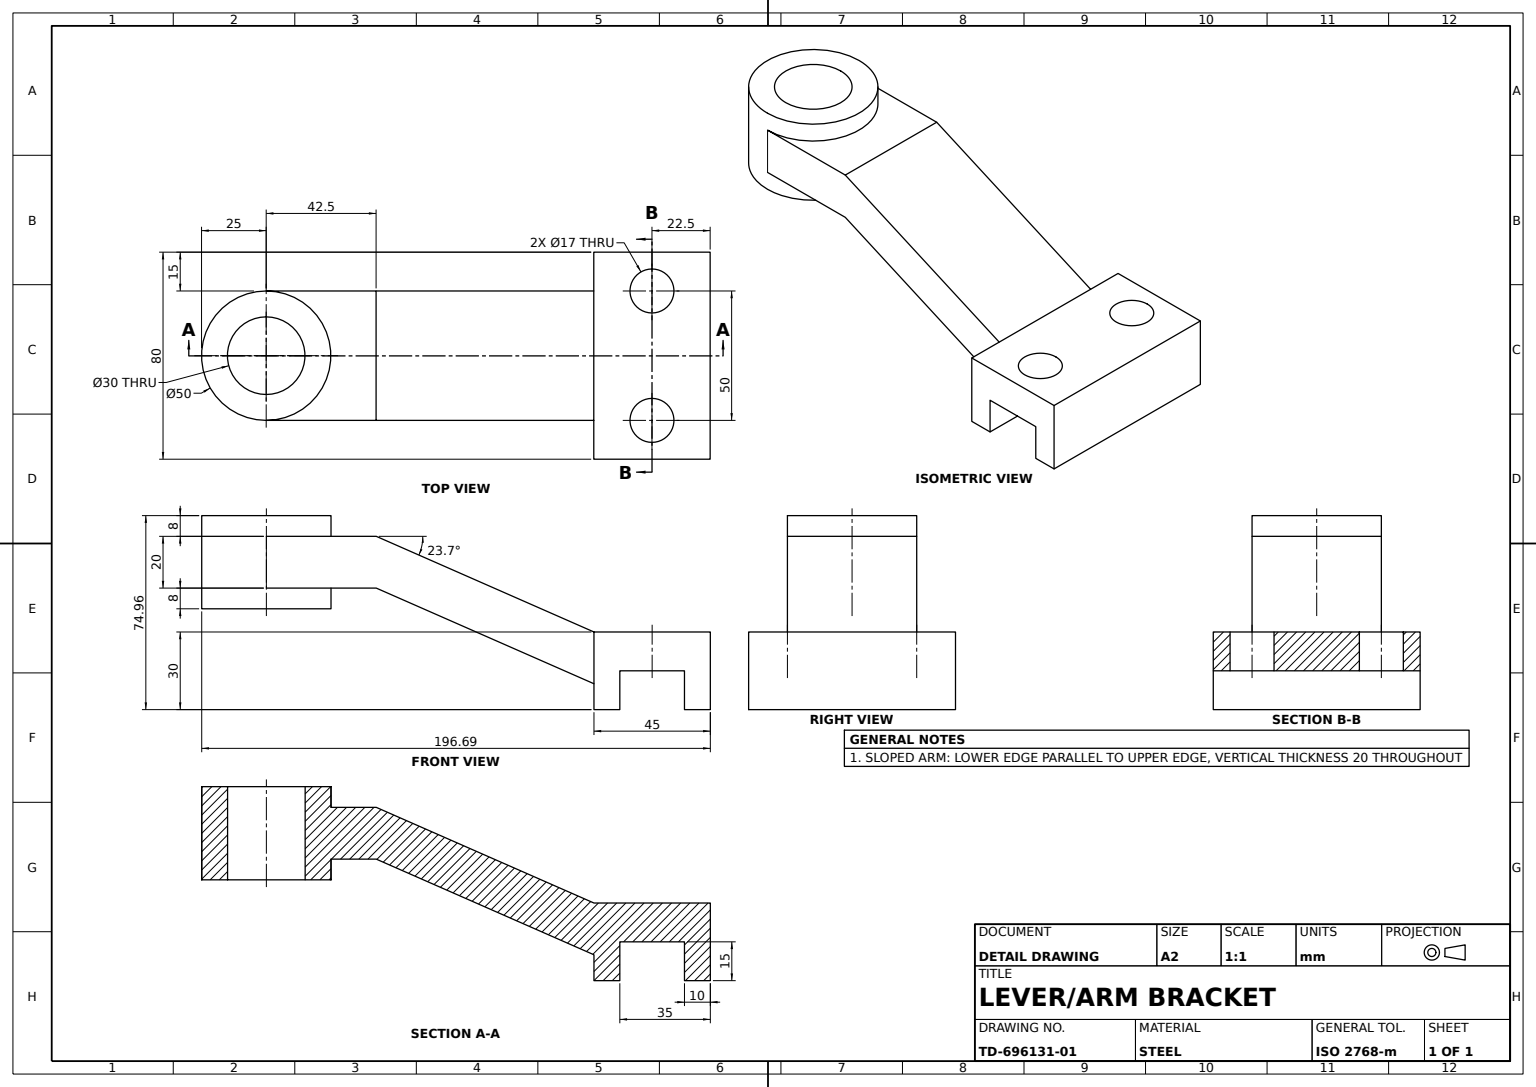
SolidWorks part; units mm, degrees
material "Plain Carbon Steel"
ref_plane "Front Plane" through (0, 0, 0) normal (0, 0, 1) x (1, 0, 0)
ref_plane "Top Plane" through (0, 0, 0) normal (0, 1, 0) x (1, 0, 0)
ref_plane "Right Plane" through (0, 0, 0) normal (1, 0, 0) x (0, 0, -1)
sketch "Arm Profile Sketch" plane through (0, 0, 0) normal (0, 0, 1) x (1, 0, 0)
  line L0 (0, 0) -> (10, 0)
  line L1 (10, 0) -> (10, 15)
  line L2 (10, 15) -> (35, 15)
  line L3 (35, 15) -> (35, 0)
  line L4 (35, 0) -> (45, 0)
  line L5 (45, 0) -> (45, 30)
  line L6 (45, 30) -> (0, 30)
  line L7 (0, 30) -> (0, 0)
  dimension "D1" = 10
  dimension "D2" = 35
  dimension "D3" = 15
  dimension "D4" = 30
extrude "Arm Body" add sketch "Arm Profile Sketch" along normal blind 80
sketch "End Block Sketch" plane through (0, 0, 80) normal (0, 0, 1) x (1, 0, 0)
  line L0 (0, 30) -> (0, 0) construction
  line L1 (0, 0) -> (10, 0) construction
  line L2 (-102.5, 75) -> (-102.5, 55)
  line L3 (-102.5, 75) -> (0, 30)
  line L4 (0, 30) -> (0, 10)
  line L5 (0, 10) -> (-102.5, 55)
  dimension "D1" = 102.5
  dimension "D2" = 10
  dimension "D3" = 55
extrude "End Block" add sketch "End Block Sketch" against normal blind 60
sketch "End Block Slot Sketch" plane through (0, 0, 80) normal (0, 0, 1) x (1, 0, 0)
  line L0 (-102.5, 75) -> (0, 30)
  line L1 (0, 30) -> (0, 10)
  line L2 (0, 10) -> (-102.5, 55)
  line L3 (-102.5, 55) -> (-102.5, 75)
extrude "End Block Slot Cut" cut sketch "End Block Slot Sketch" against normal blind 15
sketch "End Block Pad Sketch" plane through (0, 0, 20) normal (0, 0, -1) x (-1, 0, 0)
  line L0 (0, 30) -> (102.5, 75)
  line L1 (102.5, 75) -> (102.5, 55)
  line L2 (102.5, 55) -> (0, 10)
  line L3 (0, 10) -> (0, 30)
extrude "End Block Pad 5mm" add sketch "End Block Pad Sketch" along normal blind 5
sketch "Mounting Holes Sketch" plane through (0, 30, 0) normal (0, 1, 0) x (1, 0, 0)
  line L0 (45, -80) -> (45, 0) construction
  line L1 (45, 0) -> (0, 0) construction
  line L2 (45, -80) -> (0, -80) construction
  circle A0 centre (22.5, -15) radius 8.5
  circle A1 centre (22.5, -65) radius 8.5
  dimension "D1" = 17
  dimension "D2" = 17
  dimension "D7" = 17
  dimension "D3" = 22.5
  dimension "D4" = 22.5
  dimension "D5" = 15
  dimension "D6" = 15
extrude "Mounting Holes 2x" cut sketch "Mounting Holes Sketch" against normal blind 15
sketch "Arm Relief Cut Sketch" plane through (0, 0, 65) normal (0, 0, 1) x (1, 0, 0)
  line L0 (-102.5, 75) -> (-84.1871, 66.9602)
  line L1 (0, 30) -> (-102.5, 75) construction
  line L2 (-84.1871, 66.9602) -> (-84.1871, 46.9602)
  line L3 (-102.5, 55) -> (0, 10) construction
  line L4 (-84.1871, 46.9602) -> (-102.5, 55)
  line L5 (-102.5, 55) -> (-102.5, 75)
extrude "Arm Relief Cut" cut sketch "Arm Relief Cut Sketch" against normal blind 55
sketch "Arm Web Sketch" plane through (0, 0, 65) normal (0, 0, 1) x (1, 0, 0)
  line L0 (-84.1871, 66.9602) -> (-126.6871, 66.9602)
  line L1 (-126.6871, 66.9602) -> (-126.6871, 46.9602)
  line L2 (-126.6871, 46.9602) -> (-84.1871, 46.9602)
  line L3 (-84.1871, 46.9602) -> (-84.1871, 66.9602)
  line L4 (-84.1871, 46.9602) -> (-84.1871, 66.9602) construction
  dimension "D1" = 42.5
extrude "Arm Web" add sketch "Arm Web Sketch" against normal blind 50
sketch "Hub Flange Lower Sketch" plane through (0, 66.9602, 0) normal (0, 1, 0) x (1, 0, 0)
  line L0 (-126.6871, -15) -> (-126.6871, -65) construction
  circle A0 centre (-126.6871, -40) radius 25
  dimension "D1" = 50
  dimension "D2" = 50
extrude "Hub Flange Lower Ø50" add sketch "Hub Flange Lower Sketch" along normal blind 8
sketch "Hub Body Sketch" plane through (0, 66.9602, 0) normal (0, -1, 0) x (1, 0, 0)
  line L0 (-126.6871, 65) -> (-126.6871, 15)
  arc A0 (-126.6871, 65) -> (-126.6871, 15) centre (-126.6871, 40) ccw
  dimension "D1" = 50
extrude "Hub Body" add sketch "Hub Body Sketch" along normal blind 20
sketch "Hub Flange Upper Sketch" plane through (0, 46.9602, 0) normal (0, -1, 0) x (1, 0, 0)
  circle A0 centre (-126.6871, 40) radius 25
  dimension "D1" = 50
  dimension "D2" = 50
extrude "Hub Flange Upper Ø50" add sketch "Hub Flange Upper Sketch" along normal blind 8
sketch "Hub Bore Sketch" plane through (0, 74.9602, 0) normal (0, 1, 0) x (1, 0, 0)
  circle A2 centre (-126.6871, -40) radius 15
  dimension "D1" = 30
  dimension "D3" = 30
extrude "Hub Bore Ø30" cut sketch "Hub Bore Sketch" against normal blind 40
